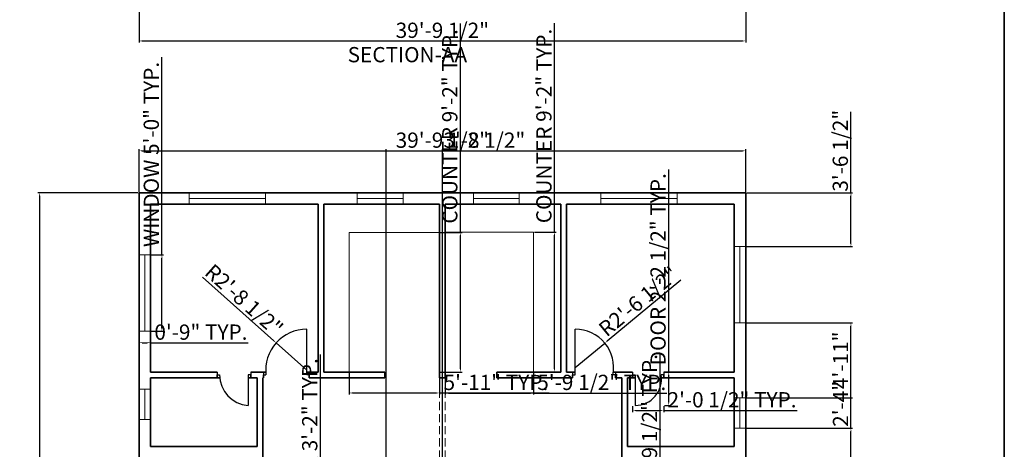
# Model space of a CAD drawing. Units: inches. Extents: x 2142 to 3604, y 1690 to 2981.
# Tile 6 of 9: x 2829 to 3604, y 2207 to 2545. Entities that reach past the tile are written whole.
import ezdxf

# ---------------------------------------------------------------- set-up
doc = ezdxf.new("R2010")
doc.units = ezdxf.units.IN
doc.linetypes.add('DASHED2', pattern=[9.525, 6.35, -3.175])
for name, color, linetype, lineweight in [('A-ANNO-DIMS', 2, 'Continuous', 18), ('A-ANNO-TEXT', 7, 'Continuous', 18), ('A-ANNO-TTLB', 7, 'Continuous', 35), ('A-DOOR', 4, 'Continuous', 25), ('A-FLOR-FIXT', 8, 'Continuous', 18), ('A-GLAZ', 4, 'Continuous', 18), ('A-WALL', 7, 'Continuous', 35), ('A-WALL-OVHD', 254, 'DASHED2', 18)]:
    doc.layers.add(name, color=color, linetype=linetype, lineweight=lineweight)
doc.styles.get("Standard").update_dxf_attribs({"font": 'arial.ttf'})
doc.dimstyles.new('ISO-25', dxfattribs={"dimtxt": 12, "dimasz": 2.5, "dimexe": 1.25, "dimexo": 0.625, "dimtad": 1, "dimdec": 0, "dimlunit": 3, "dimtxsty": 'Standard', "dimcen": 2.5, "dimadec": 0, "dimazin": 0, "dimtfac": 1, "dimtdec": 0, "dimtmove": 0, "dimatfit": 3, "dimfxl": 1, "dimarcsym": 0})

# ---------------------------------------------------------------- blocks, each defined once
blk = doc.blocks.new('DOOR-BED-REAR-L')
for p, q in [((34.09, 2.25), (34.09, 38.25)), ((0, 4.5), (0, 0)), ((0, 0), (0, 2.25)), ((0, 2.25), (2, 2.25)), ((36.09, 2.25), (34.09, 2.25)), ((36.09, 4.5), (36.09, 0)), ((36.09, 0), (36.09, 2.25))]:
    blk.add_line(p, q)
blk.add_arc((34.09, 5.95), 32.3, 90, 186.57373)
blk = doc.blocks.new('DOOR-BED-REAR-R')
for p, q in [((2, 2.25), (2, 38.25)), ((0, 4.5), (0, 0)), ((0, 0), (0, 2.25)), ((0, 2.25), (2, 2.25)), ((33.74, 2.25), (31.74, 2.25)), ((33.74, 4.5), (33.74, 0)), ((33.74, 0), (33.74, 2.25))]:
    blk.add_line(p, q)
blk.add_arc((2, 7.96), 30.29, 349.12785, 90)
blk = doc.blocks.new('DOOR-BATH-REAR-R')
for p, q in [((0, 26.25), (0, 21.75)), ((0, 21.75), (0, 24)), ((0, 24), (2, 24)), ((2, 24), (2, 0)), ((24.48, 24), (22.48, 24)), ((24.48, 26.25), (24.48, 21.75)), ((24.48, 21.75), (24.48, 24))]:
    blk.add_line(p, q)
blk.add_arc((2, 20.74), 20.74, 270, 9.03962)
blk = doc.blocks.new('DOOR-BATH-REAR-L')
for p, q in [((0, 26.25), (0, 21.75)), ((0, 21.75), (0, 24)), ((0, 24), (2, 24)), ((26.43, 24), (24.43, 24)), ((24.43, 24), (24.43, 0)), ((26.43, 26.25), (26.43, 21.75)), ((26.43, 21.75), (26.43, 24))]:
    blk.add_line(p, q)
blk.add_arc((26.05, 24), 24.05, 180, 266.13759)
blk = doc.blocks.new('COUNTER-KITCHEN-L')
for p, q in [((0, 0), (0, 109.77)), ((0, 109.77), (71.11, 109.77))]:
    blk.add_line(p, q)
blk = doc.blocks.new('COUNTER-KITCHEN-R')
for p, q in [((0, 110.14), (69.54, 110.14)), ((69.54, 110.14), (69.54, 0))]:
    blk.add_line(p, q)
blk = doc.blocks.new('WINDOW-60')
for p, q in [((0, 60), (9, 60)), ((9, 60), (4.5, 60)), ((4.5, 60), (4.5, 0)), ((4.5, 0), (0, 0)), ((0, 0), (9, 0))]:
    blk.add_line(p, q)
blk = doc.blocks.new('WINDOW-24')
for p, q in [((0, 24), (9, 24)), ((9, 24), (4.5, 24)), ((4.5, 24), (4.5, 0)), ((4.5, 0), (0, 0)), ((0, 0), (9, 0))]:
    blk.add_line(p, q)
blk = doc.blocks.new('WINDOW-24-B')
for p, q in [((4.5, 24), (0, 24)), ((0, 24), (9, 24)), ((4.5, 0), (4.5, 24)), ((4.5, 24), (4.5, 24)), ((0, 0), (9, 0)), ((9, 0), (4.5, 0)), ((4.5, 0), (4.5, 0))]:
    blk.add_line(p, q)
blk = doc.blocks.new('WINDOW-36')
for p, q in [((0, 9), (0, 0)), ((36, 4.5), (36, 9)), ((36, 9), (36, 0)), ((0, 0), (0, 4.5)), ((0, 4.5), (36, 4.5))]:
    blk.add_line(p, q)
blk = doc.blocks.new('WINDOW-60-B')
for p, q in [((4.5, 60), (0, 60)), ((0, 60), (9, 60)), ((4.5, 0), (4.5, 60)), ((9, 0), (0, 0)), ((0, 0), (4.5, 0))]:
    blk.add_line(p, q)
blk = doc.blocks.new('*D37')
at = {"layer": 'A-ANNO-DIMS', "color": 0, "lineweight": -2, "transparency": 16777216}
for p, q in [((2941.33, 2359.65), (2941.33, 2515.25)), ((2932.96, 2359.65), (2942.58, 2359.65)), ((2941.33, 2302.15), (2941.33, 2357.15)), ((2932.96, 2299.65), (2942.58, 2299.65))]:
    blk.add_line(p, q, dxfattribs=at)
at = {"layer": 'A-ANNO-DIMS', "color": 0, "transparency": 16777216}
for points in [[(2940.92, 2357.15), (2941.75, 2357.15), (2941.33, 2359.65)], [(2940.92, 2302.15), (2941.75, 2302.15), (2941.33, 2299.65)]]:
    blk.add_solid(points, dxfattribs=at)
at = {"layer": 'Defpoints', "color": 0, "transparency": 16777216}
for p in [(2932.33, 2359.65), (2941.33, 2359.65), (2932.33, 2299.65)]:
    blk.add_point(p, dxfattribs=at)
at = {"layer": 'A-ANNO-DIMS', "color": 0, "transparency": 16777216, "insert": (2934.5, 2438.7), "char_height": 12, "attachment_point": 5, "rotation": 90}
blk.add_mtext('WINDOW 5\'-0" TYP.', dxfattribs=at)
blk = doc.blocks.new('*D38')
at = {"layer": 'A-ANNO-DIMS', "color": 0, "lineweight": -2, "transparency": 16777216}
for p, q in [((2923.33, 2299.03), (2923.33, 2289.4)), ((2932.33, 2299.03), (2932.33, 2289.4)), ((2925.83, 2290.65), (2929.83, 2290.65)), ((2932.33, 2290.65), (3009.23, 2290.65))]:
    blk.add_line(p, q, dxfattribs=at)
at = {"layer": 'A-ANNO-DIMS', "color": 0, "transparency": 16777216}
for points in [[(2925.83, 2291.07), (2925.83, 2290.24), (2923.33, 2290.65)], [(2929.83, 2291.07), (2929.83, 2290.24), (2932.33, 2290.65)]]:
    blk.add_solid(points, dxfattribs=at)
at = {"layer": 'Defpoints', "color": 0, "transparency": 16777216}
for p in [(2923.33, 2299.65), (2932.33, 2299.65), (2932.33, 2290.65)]:
    blk.add_point(p, dxfattribs=at)
at = {"layer": 'A-ANNO-DIMS', "color": 0, "transparency": 16777216, "insert": (2972.03, 2297.41), "char_height": 12, "attachment_point": 5}
blk.add_mtext('0\'-9" TYP.', dxfattribs=at)
blk = doc.blocks.new('*D49')
at = {"layer": 'A-ANNO-DIMS', "color": 0, "lineweight": -2, "transparency": 16777216}
for p, q in [((3340.24, 2267.56), (3340.24, 2426.77)), ((3336.93, 2267.56), (3341.49, 2267.56)), ((3340.24, 2243.81), (3340.24, 2265.06)), ((3336.93, 2241.31), (3341.49, 2241.31))]:
    blk.add_line(p, q, dxfattribs=at)
at = {"layer": 'A-ANNO-DIMS', "color": 0, "transparency": 16777216}
for points in [[(3339.83, 2265.06), (3340.66, 2265.06), (3340.24, 2267.56)], [(3339.83, 2243.81), (3340.66, 2243.81), (3340.24, 2241.31)]]:
    blk.add_solid(points, dxfattribs=at)
at = {"layer": 'Defpoints', "color": 0, "transparency": 16777216}
for p in [(3336.31, 2267.56), (3340.24, 2267.56), (3336.31, 2241.31)]:
    blk.add_point(p, dxfattribs=at)
at = {"layer": 'A-ANNO-DIMS', "color": 0, "transparency": 16777216, "insert": (3333.41, 2348.41), "char_height": 12, "attachment_point": 5, "rotation": 90}
blk.add_mtext('DOOR 2\'-2 1/2" TYP.', dxfattribs=at)
blk = doc.blocks.new('*D50')
at = {"layer": 'A-ANNO-DIMS', "color": 0, "lineweight": -2, "transparency": 16777216}
for p, q in [((3311.82, 2240.68), (3311.82, 2236.12)), ((3336.31, 2240.68), (3336.31, 2236.12)), ((3314.32, 2237.37), (3333.81, 2237.37)), ((3336.31, 2237.37), (3441.37, 2237.37))]:
    blk.add_line(p, q, dxfattribs=at)
at = {"layer": 'A-ANNO-DIMS', "color": 0, "transparency": 16777216}
for points in [[(3314.32, 2237.79), (3314.32, 2236.95), (3311.82, 2237.37)], [(3333.81, 2237.79), (3333.81, 2236.95), (3336.31, 2237.37)]]:
    blk.add_solid(points, dxfattribs=at)
at = {"layer": 'Defpoints', "color": 0, "transparency": 16777216}
for p in [(3311.82, 2241.31), (3336.31, 2241.31), (3336.31, 2237.37)]:
    blk.add_point(p, dxfattribs=at)
at = {"layer": 'A-ANNO-DIMS', "color": 0, "transparency": 16777216, "insert": (3390.09, 2244.2), "char_height": 12, "attachment_point": 5}
blk.add_mtext('2\'-0 1/2" TYP.', dxfattribs=at)
blk = doc.blocks.new('*D54')
at = {"layer": 'A-ANNO-DIMS', "color": 0, "lineweight": -2, "transparency": 16777216}
for p, q in [((3333.52, 2177.88), (3333.52, 2281.61)), ((3330.21, 2177.88), (3334.77, 2177.88)), ((3333.52, 2158.66), (3333.52, 2175.38)), ((3330.21, 2156.16), (3334.77, 2156.16))]:
    blk.add_line(p, q, dxfattribs=at)
at = {"layer": 'A-ANNO-DIMS', "color": 0, "transparency": 16777216}
for points in [[(3333.1, 2175.38), (3333.94, 2175.38), (3333.52, 2177.88)], [(3333.1, 2158.66), (3333.94, 2158.66), (3333.52, 2156.16)]]:
    blk.add_solid(points, dxfattribs=at)
at = {"layer": 'Defpoints', "color": 0, "transparency": 16777216}
for p in [(3329.58, 2177.88), (3333.52, 2177.88), (3329.58, 2156.16)]:
    blk.add_point(p, dxfattribs=at)
at = {"layer": 'A-ANNO-DIMS', "color": 0, "transparency": 16777216, "insert": (3326.69, 2231), "char_height": 12, "attachment_point": 5, "rotation": 90}
blk.add_mtext('1\'-9 1/2" TYP.', dxfattribs=at)
blk = doc.blocks.new('*D55')
at = {"layer": 'A-ANNO-DIMS', "color": 0, "lineweight": -2, "transparency": 16777216}
for p, q in [((3066.08, 2150.15), (3066.08, 2281.4)), ((3061, 2150.15), (3067.33, 2150.15)), ((3066.08, 2114.61), (3066.08, 2147.65)), ((3061, 2112.11), (3067.33, 2112.11))]:
    blk.add_line(p, q, dxfattribs=at)
at = {"layer": 'A-ANNO-DIMS', "color": 0, "transparency": 16777216}
for points in [[(3065.66, 2147.65), (3066.5, 2147.65), (3066.08, 2150.15)], [(3065.66, 2114.61), (3066.5, 2114.61), (3066.08, 2112.11)]]:
    blk.add_solid(points, dxfattribs=at)
at = {"layer": 'Defpoints', "color": 0, "transparency": 16777216}
for p in [(3060.37, 2150.15), (3066.08, 2150.15), (3060.37, 2112.11)]:
    blk.add_point(p, dxfattribs=at)
at = {"layer": 'A-ANNO-DIMS', "color": 0, "transparency": 16777216, "insert": (3059.24, 2217.03), "char_height": 12, "attachment_point": 5, "rotation": 90}
blk.add_mtext('DOOR 3\'-2" TYP.', dxfattribs=at)
blk = doc.blocks.new('*D67')
at = {"layer": 'A-ANNO-DIMS', "color": 0, "lineweight": -2, "transparency": 16777216}
for p, q in [((3176.3, 2377.33), (3176.3, 2541.63)), ((3160.46, 2377.33), (3177.55, 2377.33)), ((3176.3, 2270.06), (3176.3, 2374.83)), ((3160.46, 2267.56), (3177.55, 2267.56))]:
    blk.add_line(p, q, dxfattribs=at)
at = {"layer": 'A-ANNO-DIMS', "color": 0, "transparency": 16777216}
for points in [[(3175.88, 2374.83), (3176.71, 2374.83), (3176.3, 2377.33)], [(3175.88, 2270.06), (3176.71, 2270.06), (3176.3, 2267.56)]]:
    blk.add_solid(points, dxfattribs=at)
at = {"layer": 'Defpoints', "color": 0, "transparency": 16777216}
for p in [(3159.83, 2377.33), (3176.3, 2377.33), (3159.83, 2267.56)]:
    blk.add_point(p, dxfattribs=at)
at = {"layer": 'A-ANNO-DIMS', "color": 0, "transparency": 16777216, "insert": (3169.46, 2460.73), "char_height": 12, "attachment_point": 5, "rotation": 90}
blk.add_mtext('COUNTER 9\'-2" TYP.', dxfattribs=at)
blk = doc.blocks.new('*D68')
at = {"layer": 'A-ANNO-DIMS', "color": 0, "lineweight": -2, "transparency": 16777216}
for p, q in [((3088.72, 2266.93), (3088.72, 2249.84)), ((3159.83, 2266.93), (3159.83, 2249.84)), ((3091.22, 2251.09), (3157.33, 2251.09)), ((3159.83, 2251.09), (3246.05, 2251.09))]:
    blk.add_line(p, q, dxfattribs=at)
at = {"layer": 'A-ANNO-DIMS', "color": 0, "transparency": 16777216}
for points in [[(3091.22, 2251.51), (3091.22, 2250.68), (3088.72, 2251.09)], [(3157.33, 2251.51), (3157.33, 2250.68), (3159.83, 2251.09)]]:
    blk.add_solid(points, dxfattribs=at)
at = {"layer": 'Defpoints', "color": 0, "transparency": 16777216}
for p in [(3088.72, 2267.56), (3159.83, 2267.56), (3159.83, 2251.09)]:
    blk.add_point(p, dxfattribs=at)
at = {"layer": 'A-ANNO-DIMS', "color": 0, "transparency": 16777216, "insert": (3204.19, 2257.85), "char_height": 12, "attachment_point": 5}
blk.add_mtext('5\'-11" TYP.', dxfattribs=at)
blk = doc.blocks.new('*D69')
at = {"layer": 'A-ANNO-DIMS', "color": 0, "lineweight": -2, "transparency": 16777216}
for p, q in [((3250.39, 2377.7), (3250.39, 2542)), ((3234.49, 2377.7), (3251.64, 2377.7)), ((3250.39, 2270.06), (3250.39, 2375.2)), ((3234.49, 2267.56), (3251.64, 2267.56))]:
    blk.add_line(p, q, dxfattribs=at)
at = {"layer": 'A-ANNO-DIMS', "color": 0, "transparency": 16777216}
for points in [[(3249.97, 2375.2), (3250.81, 2375.2), (3250.39, 2377.7)], [(3249.97, 2270.06), (3250.81, 2270.06), (3250.39, 2267.56)]]:
    blk.add_solid(points, dxfattribs=at)
at = {"layer": 'Defpoints', "color": 0, "transparency": 16777216}
for p in [(3233.87, 2377.7), (3250.39, 2377.7), (3233.87, 2267.56)]:
    blk.add_point(p, dxfattribs=at)
at = {"layer": 'A-ANNO-DIMS', "color": 0, "transparency": 16777216, "insert": (3243.56, 2461.1), "char_height": 12, "attachment_point": 5, "rotation": 90}
blk.add_mtext('COUNTER 9\'-2" TYP.', dxfattribs=at)
blk = doc.blocks.new('*D70')
at = {"layer": 'A-ANNO-DIMS', "color": 0, "lineweight": -2, "transparency": 16777216}
for p, q in [((3164.33, 2266.93), (3164.33, 2249.79)), ((3233.87, 2266.93), (3233.87, 2249.79)), ((3166.83, 2251.04), (3231.37, 2251.04)), ((3233.87, 2251.04), (3338.73, 2251.04))]:
    blk.add_line(p, q, dxfattribs=at)
at = {"layer": 'A-ANNO-DIMS', "color": 0, "transparency": 16777216}
for points in [[(3166.83, 2251.45), (3166.83, 2250.62), (3164.33, 2251.04)], [(3231.37, 2251.45), (3231.37, 2250.62), (3233.87, 2251.04)]]:
    blk.add_solid(points, dxfattribs=at)
at = {"layer": 'Defpoints', "color": 0, "transparency": 16777216}
for p in [(3164.33, 2267.56), (3233.87, 2267.56), (3233.87, 2251.04)]:
    blk.add_point(p, dxfattribs=at)
at = {"layer": 'A-ANNO-DIMS', "color": 0, "transparency": 16777216, "insert": (3287.55, 2257.87), "char_height": 12, "attachment_point": 5}
blk.add_mtext('5\'-9 1/2" TYP.', dxfattribs=at)
blk = doc.blocks.new('*D77')
at = {"layer": 'A-ANNO-DIMS', "color": 0, "lineweight": -2, "transparency": 16777216}
for p, q in [((2923.33, 2409.18), (2923.33, 2442.81)), ((2925.83, 2441.56), (3398.33, 2441.56)), ((3400.83, 2409.18), (3400.83, 2442.81))]:
    blk.add_line(p, q, dxfattribs=at)
at = {"layer": 'A-ANNO-DIMS', "color": 0, "transparency": 16777216}
for points in [[(2925.83, 2441.98), (2925.83, 2441.14), (2923.33, 2441.56)], [(3398.33, 2441.98), (3398.33, 2441.14), (3400.83, 2441.56)]]:
    blk.add_solid(points, dxfattribs=at)
at = {"layer": 'Defpoints', "color": 0, "transparency": 16777216}
for p in [(3400.83, 2441.56), (2923.33, 2408.56), (3400.83, 2408.56)]:
    blk.add_point(p, dxfattribs=at)
at = {"layer": 'A-ANNO-DIMS', "color": 0, "transparency": 16777216, "insert": (3162.08, 2448.39), "char_height": 12, "attachment_point": 5}
blk.add_mtext('39\'-9 1/2"', dxfattribs=at)
blk = doc.blocks.new('*D78')
at = {"layer": 'A-ANNO-DIMS', "color": 0, "lineweight": -2, "transparency": 16777216}
for p, q in [((2922.71, 2408.56), (2843.63, 2408.56)), ((2844.88, 2406.06), (2844.88, 1797.04)), ((3112.57, 1794.54), (2843.63, 1794.54))]:
    blk.add_line(p, q, dxfattribs=at)
at = {"layer": 'A-ANNO-DIMS', "color": 0, "transparency": 16777216}
for points in [[(2844.46, 2406.06), (2845.3, 2406.06), (2844.88, 2408.56)], [(2844.46, 1797.04), (2845.3, 1797.04), (2844.88, 1794.54)]]:
    blk.add_solid(points, dxfattribs=at)
at = {"layer": 'Defpoints', "color": 0, "transparency": 16777216}
for p in [(2923.33, 2408.56), (2844.88, 1794.54), (3113.2, 1794.54)]:
    blk.add_point(p, dxfattribs=at)
at = {"layer": 'A-ANNO-DIMS', "color": 0, "transparency": 16777216, "insert": (2838.13, 2101.55), "char_height": 12, "attachment_point": 5, "rotation": 90}
blk.add_mtext('51\'-2"', dxfattribs=at)
blk = doc.blocks.new('*D93')
at = {"layer": 'A-ANNO-DIMS', "color": 0, "lineweight": -2, "transparency": 16777216}
for p, q in [((2923.33, 2560.39), (2923.33, 2526.72)), ((3400.83, 2560.39), (3400.83, 2526.72)), ((2925.83, 2527.97), (3398.33, 2527.97))]:
    blk.add_line(p, q, dxfattribs=at)
at = {"layer": 'A-ANNO-DIMS', "color": 0, "transparency": 16777216}
for points in [[(2925.83, 2528.38), (2925.83, 2527.55), (2923.33, 2527.97)], [(3398.33, 2528.38), (3398.33, 2527.55), (3400.83, 2527.97)]]:
    blk.add_solid(points, dxfattribs=at)
at = {"layer": 'Defpoints', "color": 0, "transparency": 16777216}
for p in [(2923.33, 2561.02), (3400.83, 2561.02), (3400.83, 2527.97)]:
    blk.add_point(p, dxfattribs=at)
at = {"layer": 'A-ANNO-DIMS', "color": 0, "transparency": 16777216, "insert": (3162.08, 2534.8), "char_height": 12, "attachment_point": 5}
blk.add_mtext('39\'-9 1/2"', dxfattribs=at)
blk = doc.blocks.new('*D112')
at = {"layer": 'A-ANNO-DIMS', "color": 0, "lineweight": -2, "transparency": 16777216}
for p, q in [((3117.83, 1878.18), (3117.83, 2442.81)), ((3120.33, 2441.56), (3159.58, 2441.56)), ((3162.08, 1878.18), (3162.08, 2442.81)), ((3162.08, 2441.56), (3225.69, 2441.56))]:
    blk.add_line(p, q, dxfattribs=at)
at = {"layer": 'A-ANNO-DIMS', "color": 0, "transparency": 16777216}
for points in [[(3120.33, 2441.98), (3120.33, 2441.14), (3117.83, 2441.56)], [(3159.58, 2441.98), (3159.58, 2441.14), (3162.08, 2441.56)]]:
    blk.add_solid(points, dxfattribs=at)
at = {"layer": 'Defpoints', "color": 0, "transparency": 16777216}
for p in [(3162.08, 2441.56), (3117.83, 1877.56), (3162.08, 1877.56)]:
    blk.add_point(p, dxfattribs=at)
at = {"layer": 'A-ANNO-DIMS', "color": 0, "transparency": 16777216, "insert": (3195.13, 2448.39), "char_height": 12, "attachment_point": 5}
blk.add_mtext('3\'-8 1/2"', dxfattribs=at)
blk = doc.blocks.new('*D120')
at = {"layer": 'A-ANNO-DIMS', "color": 0, "lineweight": -2, "transparency": 16777216}
for p, q in [((3483.7, 2223.37), (3483.7, 2259.22)), ((3401.46, 2223.37), (3484.95, 2223.37)), ((3483.7, 2197.99), (3483.7, 2220.87)), ((3401.46, 2195.49), (3484.95, 2195.49))]:
    blk.add_line(p, q, dxfattribs=at)
at = {"layer": 'A-ANNO-DIMS', "color": 0, "transparency": 16777216}
for points in [[(3483.29, 2220.87), (3484.12, 2220.87), (3483.7, 2223.37)], [(3483.29, 2197.99), (3484.12, 2197.99), (3483.7, 2195.49)]]:
    blk.add_solid(points, dxfattribs=at)
at = {"layer": 'Defpoints', "color": 0, "transparency": 16777216}
for p in [(3400.83, 2223.37), (3483.7, 2223.37), (3400.83, 2195.49)]:
    blk.add_point(p, dxfattribs=at)
at = {"layer": 'A-ANNO-DIMS', "color": 0, "transparency": 16777216, "insert": (3477.06, 2242.54), "char_height": 12, "attachment_point": 5, "rotation": 90}
blk.add_mtext('2\'-4"', dxfattribs=at)
blk = doc.blocks.new('*D121')
at = {"layer": 'A-ANNO-DIMS', "color": 0, "lineweight": -2, "transparency": 16777216}
for p, q in [((3401.46, 2306.21), (3484.95, 2306.21)), ((3483.7, 2249.87), (3483.7, 2303.71)), ((3401.46, 2247.37), (3484.95, 2247.37))]:
    blk.add_line(p, q, dxfattribs=at)
at = {"layer": 'A-ANNO-DIMS', "color": 0, "transparency": 16777216}
for points in [[(3483.29, 2303.71), (3484.12, 2303.71), (3483.7, 2306.21)], [(3483.29, 2249.87), (3484.12, 2249.87), (3483.7, 2247.37)]]:
    blk.add_solid(points, dxfattribs=at)
at = {"layer": 'Defpoints', "color": 0, "transparency": 16777216}
for p in [(3400.83, 2306.21), (3483.7, 2306.21), (3400.83, 2247.37)]:
    blk.add_point(p, dxfattribs=at)
at = {"layer": 'A-ANNO-DIMS', "color": 0, "transparency": 16777216, "insert": (3477.06, 2276.79), "char_height": 12, "attachment_point": 5, "rotation": 90}
blk.add_mtext('4\'-11"', dxfattribs=at)
blk = doc.blocks.new('*D122')
at = {"layer": 'A-ANNO-DIMS', "color": 0, "lineweight": -2, "transparency": 16777216}
for p, q in [((3483.7, 2408.56), (3483.7, 2472.16)), ((3401.46, 2408.56), (3484.95, 2408.56)), ((3483.7, 2368.71), (3483.7, 2406.06)), ((3401.46, 2366.21), (3484.95, 2366.21))]:
    blk.add_line(p, q, dxfattribs=at)
at = {"layer": 'A-ANNO-DIMS', "color": 0, "transparency": 16777216}
for points in [[(3483.29, 2406.06), (3484.12, 2406.06), (3483.7, 2408.56)], [(3483.29, 2368.71), (3484.12, 2368.71), (3483.7, 2366.21)]]:
    blk.add_solid(points, dxfattribs=at)
at = {"layer": 'Defpoints', "color": 0, "transparency": 16777216}
for p in [(3400.83, 2408.56), (3483.7, 2408.56), (3400.83, 2366.21)]:
    blk.add_point(p, dxfattribs=at)
at = {"layer": 'A-ANNO-DIMS', "color": 0, "transparency": 16777216, "insert": (3476.87, 2441.61), "char_height": 12, "attachment_point": 5, "rotation": 90}
blk.add_mtext('3\'-6 1/2"', dxfattribs=at)
blk = doc.blocks.new('*D124')
at = {"layer": 'A-ANNO-DIMS', "color": 0, "lineweight": -2, "transparency": 16777216}
for p, q in [((2973.28, 2342.13), (3029.34, 2292.16)), ((3055.32, 2269.01), (3031.21, 2290.5))]:
    blk.add_line(p, q, dxfattribs=at)
at = {"layer": 'A-ANNO-DIMS', "color": 0, "transparency": 16777216}
blk.add_solid([(3029.62, 2292.47), (3029.06, 2291.85), (3031.21, 2290.5)], dxfattribs=at)
at = {"layer": 'Defpoints', "color": 0, "transparency": 16777216}
for p in [(3031.21, 2290.5), (3055.32, 2269.01)]:
    blk.add_point(p, dxfattribs=at)
at = {"layer": 'A-ANNO-DIMS', "color": 0, "transparency": 16777216, "insert": (3004.92, 2323.08), "char_height": 12, "attachment_point": 5, "rotation": 318.28787}
blk.add_mtext('R2\'-8 1/2"', dxfattribs=at)
blk = doc.blocks.new('*D126')
at = {"layer": 'A-ANNO-DIMS', "color": 0, "lineweight": -2, "transparency": 16777216}
for p, q in [((3349.78, 2339.73), (3291.89, 2291.9)), ((3266.61, 2271.02), (3289.96, 2290.31))]:
    blk.add_line(p, q, dxfattribs=at)
at = {"layer": 'A-ANNO-DIMS', "color": 0, "transparency": 16777216}
blk.add_solid([(3291.63, 2292.23), (3292.16, 2291.58), (3289.96, 2290.31)], dxfattribs=at)
at = {"layer": 'Defpoints', "color": 0, "transparency": 16777216}
for p in [(3289.96, 2290.31), (3266.61, 2271.02)]:
    blk.add_point(p, dxfattribs=at)
at = {"layer": 'A-ANNO-DIMS', "color": 0, "transparency": 16777216, "insert": (3317.45, 2321.88), "char_height": 12, "attachment_point": 5, "rotation": 39.56277}
blk.add_mtext('R2\'-6 1/2"', dxfattribs=at)

msp = doc.modelspace()

# ---------------------------------------------------------------- linework, layer by layer
at = {"layer": 'A-ANNO-TTLB'}
msp.add_lwpolyline([(2142.1, 2981.01), (3604.42, 2981.01), (3604.42, 1690.13), (2142.1, 1690.13)], close=True, dxfattribs=at)
at = {"layer": 'A-WALL'}
for p, q in [((2923.33, 2408.56), (3400.83, 2408.56)), ((2923.33, 2408.56), (3400.83, 2408.56)), ((2923.33, 2408.56), (2923.33, 1816.06)), ((3400.83, 2408.56), (3400.83, 1816.06)), ((2932.33, 2399.56), (3064.33, 2399.56)), ((2932.33, 2399.56), (2932.33, 2267.56)), ((3064.33, 2399.56), (3064.33, 2267.56)), ((3068.83, 2399.56), (3159.83, 2399.56)), ((3068.83, 2399.56), (3068.83, 2267.56)), ((3159.83, 2399.56), (3159.83, 2263.06)), ((3164.33, 2399.56), (3255.33, 2399.56)), ((3164.33, 2399.56), (3164.33, 2263.06)), ((3255.33, 2399.56), (3255.33, 2267.56)), ((3259.83, 2399.56), (3391.83, 2399.56)), ((3259.83, 2399.56), (3259.83, 2267.56)), ((3391.83, 2399.56), (3391.83, 2267.56)), ((2932.33, 2267.56), (2984.77, 2267.56)), ((3011.2, 2267.56), (3023.05, 2267.56)), ((3055.32, 2267.56), (3064.33, 2267.56)), ((3068.83, 2267.56), (3116.87, 2267.56)), ((3116.87, 2267.56), (3116.87, 2263.06)), ((3204.83, 2267.56), (3255.33, 2267.56)), ((3204.83, 2267.56), (3204.83, 2263.06)), ((3259.83, 2267.56), (3266.61, 2267.56)), ((3296.7, 2267.56), (3311.82, 2267.56)), ((3336.31, 2267.56), (3391.83, 2267.56)), ((2932.33, 2263.06), (2986.87, 2263.06)), ((2932.33, 2263.06), (2932.33, 2209.06)), ((3009.2, 2263.06), (3016.33, 2263.06)), ((3016.33, 2209.06), (3016.33, 2263.06)), ((3020.83, 2263.06), (3021.23, 2263.06)), ((3020.83, 2263.06), (3020.83, 2177.56)), ((3057.32, 2263.06), (3116.87, 2263.06)), ((3159.83, 2263.06), (3164.33, 2263.06)), ((3204.83, 2263.06), (3264.61, 2263.06)), ((3298.36, 2263.06), (3303.33, 2263.06)), ((3303.33, 2263.06), (3303.33, 2177.88)), ((3307.83, 2263.06), (3313.82, 2263.06)), ((3307.83, 2209.06), (3307.83, 2263.06)), ((3334.54, 2263.06), (3391.83, 2263.06)), ((3391.83, 2263.06), (3391.83, 2209.06)), ((2932.33, 2209.06), (3016.33, 2209.06)), ((3307.83, 2209.06), (3391.83, 2209.06))]:
    msp.add_line(p, q, dxfattribs=at)
at = {"layer": 'A-WALL-OVHD'}
for p, q in [((3159.83, 2263.06), (3159.83, 2263.06)), ((3159.83, 2263.06), (3159.83, 2151.06)), ((3164.33, 2263.06), (3164.33, 2151.06))]:
    msp.add_line(p, q, dxfattribs=at)

# ---------------------------------------------------------------- block references
at = {"layer": 'A-DOOR'}
for name, p in [('DOOR-BED-REAR-L', (3021.23, 2263.06)), ('DOOR-BED-REAR-R', (3264.61, 2263.06)), ('DOOR-BATH-REAR-L', (2984.77, 2241.31)), ('DOOR-BATH-REAR-R', (3311.82, 2241.31))]:
    msp.add_blockref(name, p, dxfattribs=at)
at = {"layer": 'A-FLOR-FIXT'}
for name, p in [('COUNTER-KITCHEN-L', (3088.72, 2267.56)), ('COUNTER-KITCHEN-R', (3164.33, 2267.56))]:
    msp.add_blockref(name, p, dxfattribs=at)
at = {"layer": 'A-GLAZ', "extrusion": (0, 0, -1), "zscale": -1}
for p, rotation in [((-3022.74, 2408.56), 270), ((-3346.93, 2408.56), 270), ((-3391.83, 2366.21), 180)]:
    msp.add_blockref('WINDOW-60', p, dxfattribs=dict(at, rotation=rotation))
at = {"layer": 'A-GLAZ'}
for name, p in [('WINDOW-36', (3095.12, 2399.56)), ('WINDOW-36', (3186.46, 2399.56)), ('WINDOW-60-B', (2923.33, 2299.65)), ('WINDOW-24', (2923.33, 2230.19)), ('WINDOW-24-B', (3391.83, 2223.37))]:
    msp.add_blockref(name, p, dxfattribs=at)

# ---------------------------------------------------------------- texts
at = {"layer": 'A-ANNO-TEXT', "insert": (3087.53, 2523.18), "char_height": 12, "attachment_point": 1}
msp.add_mtext_dynamic_manual_height_columns('SECTION-AA', width=353.6552, gutter_width=12.5, heights=[0], dxfattribs=at)

# ---------------------------------------------------------------- dimensions: what is measured, and where the dimension line sits
at = {"layer": 'A-ANNO-DIMS'}
for base, p1, p2, picture, middle in [((3400.83, 2527.97), (2923.33, 2561.02), (3400.83, 2561.02), '*D93', (3162.08, 2534.8)), ((3400.83, 2441.56), (2923.33, 2408.56), (3400.83, 2408.56), '*D77', (3162.08, 2448.39)), ((3162.083094, 2441.558519), (3117.833094, 1877.558519), (3162.083094, 1877.558519), '*D112', (3195.13442415, 2448.39225024))]:
    dim = msp.add_linear_dim(base=base, p1=p1, p2=p2, dimstyle='ISO-25', override={"dimdec": 1, "dimlfac": 1, "dimrnd": 0, "dimzin": 1, "dimdsep": 46, "dimlunit": 4, "dimfrac": 2}, dxfattribs=at)
    dim.commit()
    dim.dimension.update_dxf_attribs({"geometry": picture, "text_midpoint": middle})
for base, p1, p2, text, picture, middle in [((3176.3, 2377.33), (3159.83, 2267.56), (3159.83, 2377.33), 'COUNTER <> TYP.', '*D67', (3169.46, 2460.73)), ((3250.39, 2377.7), (3233.87, 2267.56), (3233.87, 2377.7), 'COUNTER <> TYP.', '*D69', (3243.56, 2461.1)), ((2941.33, 2359.65), (2932.33, 2299.65), (2932.33, 2359.65), 'WINDOW <> TYP.', '*D37', (2934.5, 2438.7)), ((3340.24264032, 2267.55851851), (3336.30514032, 2241.30851851), (3336.30514032, 2267.55851851), 'DOOR <> TYP.', '*D49', (3333.40890908, 2348.41339573)), ((3066.08, 2150.15), (3060.37, 2112.11), (3060.37, 2150.15), 'DOOR <> TYP.', '*D55', (3059.24, 2217.03)), ((3333.52, 2177.88), (3329.58, 2156.16), (3329.58, 2177.88), '<> TYP.', '*D54', (3326.69, 2231))]:
    dim = msp.add_linear_dim(base=base, p1=p1, p2=p2, angle=90, text=text, dimstyle='ISO-25', override={"dimdec": 1, "dimlfac": 1, "dimrnd": 0, "dimzin": 1, "dimdsep": 46, "dimlunit": 4, "dimfrac": 2}, dxfattribs=at)
    dim.commit()
    dim.dimension.update_dxf_attribs({"geometry": picture, "text_midpoint": middle})
for base, p1, p2, picture, middle in [((3483.7047, 2408.5585), (3400.8331, 2366.2098), (3400.8331, 2408.5585), '*D122', (3476.8709, 2441.6098)), ((2844.88, 1794.54), (2923.33, 2408.56), (3113.2, 1794.54), '*D78', (2838.13, 2101.55)), ((3483.7, 2306.21), (3400.83, 2247.37), (3400.83, 2306.21), '*D121', (3477.06, 2276.79)), ((3483.7, 2223.37), (3400.83, 2195.49), (3400.83, 2223.37), '*D120', (3477.06, 2242.54))]:
    dim = msp.add_linear_dim(base=base, p1=p1, p2=p2, angle=90, dimstyle='ISO-25', override={"dimdec": 1, "dimlfac": 1, "dimrnd": 0, "dimzin": 1, "dimdsep": 46, "dimlunit": 4, "dimfrac": 2}, dxfattribs=at)
    dim.commit()
    dim.dimension.update_dxf_attribs({"geometry": picture, "text_midpoint": middle})
for center, mpoint, picture, middle in [((3055.32, 2269.01), (3031.21, 2290.5), '*D124', (3004.92, 2323.08)), ((3266.61, 2271.02), (3289.96, 2290.31), '*D126', (3317.45, 2321.88))]:
    dim = msp.add_radius_dim(center=center, mpoint=mpoint, dimstyle='ISO-25', override={"dimdec": 1, "dimlfac": 1, "dimrnd": 0, "dimzin": 1, "dimdsep": 46, "dimlunit": 4, "dimfrac": 2}, dxfattribs=at)
    dim.commit()
    dim.dimension.update_dxf_attribs({"geometry": picture, "text_midpoint": middle})
for base, p1, p2, picture, middle in [((2932.33, 2290.65), (2923.33, 2299.65), (2932.33, 2299.65), '*D38', (2972.03, 2297.41)), ((3233.87, 2251.04), (3164.33, 2267.56), (3233.87, 2267.56), '*D70', (3287.55, 2257.87)), ((3159.83, 2251.09), (3088.72, 2267.56), (3159.83, 2267.56), '*D68', (3204.19, 2257.85)), ((3336.31, 2237.37), (3311.82, 2241.31), (3336.31, 2241.31), '*D50', (3390.09, 2244.2))]:
    dim = msp.add_linear_dim(base=base, p1=p1, p2=p2, text='<> TYP.', dimstyle='ISO-25', override={"dimdec": 1, "dimlfac": 1, "dimrnd": 0, "dimzin": 1, "dimdsep": 46, "dimlunit": 4, "dimfrac": 2}, dxfattribs=at)
    dim.commit()
    dim.dimension.update_dxf_attribs({"geometry": picture, "text_midpoint": middle})

doc.saveas('drawing.dxf')
